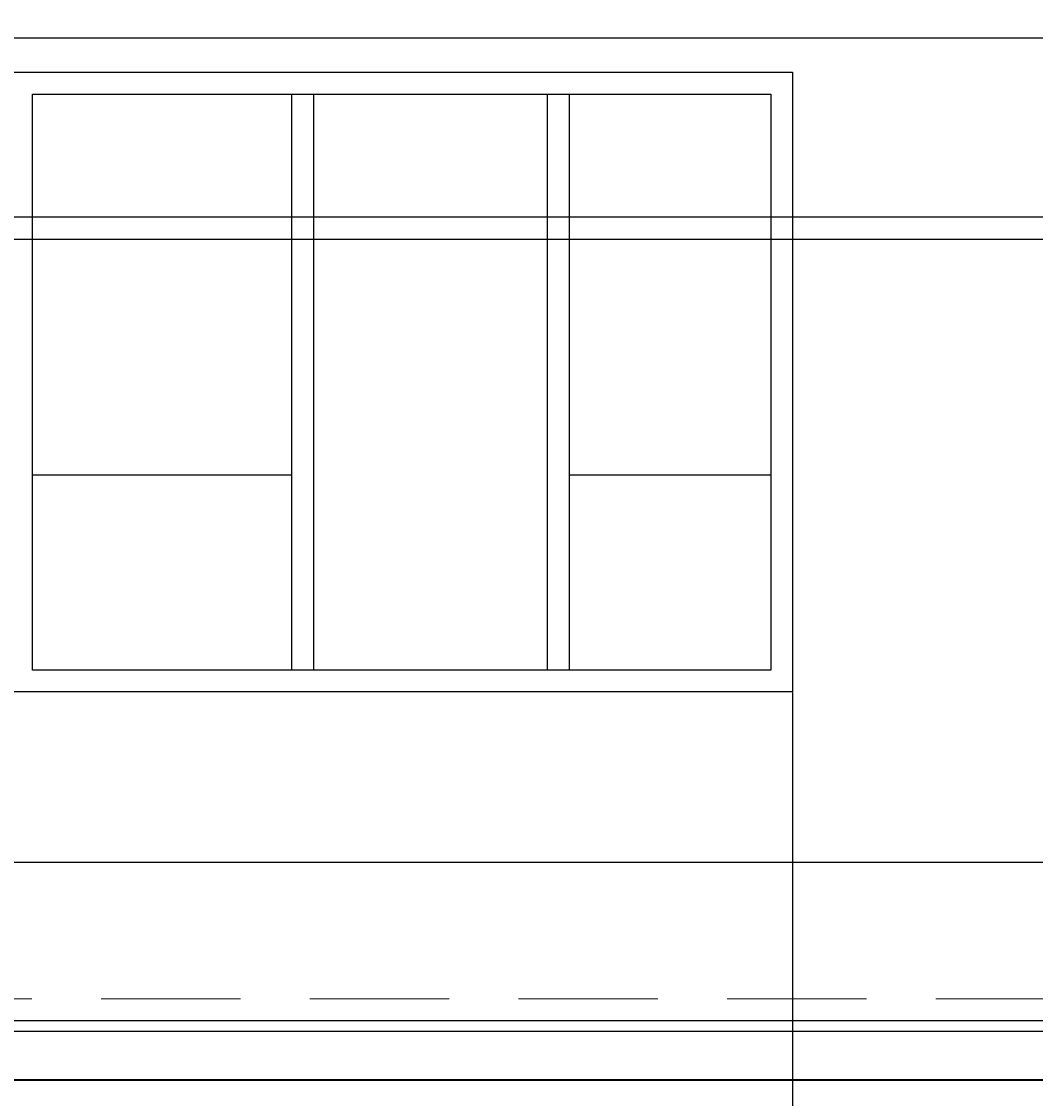
# Model space of a CAD drawing. Units: inches. Extents: x -145 to 510, y 5 to 386.
# Tile 6 of 25: x 89 to 182, y 78 to 177. Entities that reach past the tile are written whole.
import ezdxf

# ---------------------------------------------------------------- set-up
doc = ezdxf.new("R2010")
doc.units = ezdxf.units.IN
doc.header["$MEASUREMENT"] = 0
doc.linetypes.add('DASHED', pattern=[19.05, 12.7, -6.35])
for name, color, linetype, lineweight in [('A-ANNO-DIMS', 2, 'Continuous', 18), ('A-ELEV', 7, 'Continuous', 35), ('A-ELEV-HIDN', 8, 'DASHED', 18), ('A-GLAZ', 4, 'Continuous', 25)]:
    doc.layers.add(name, color=color, linetype=linetype, lineweight=lineweight)
doc.styles.get("Standard").update_dxf_attribs({"font": 'arial.ttf'})
doc.dimstyles.get("Standard").update_dxf_attribs({"dimtxt": 0.6875, "dimasz": 0.18, "dimexe": 0.18, "dimexo": 0.0625, "dimgap": 0.09, "dimtad": 0, "dimtih": 1, "dimtoh": 1, "dimdec": 4, "dimzin": 0, "dimdsep": 46, "dimlunit": 4, "dimtxsty": 'Standard', "dimcen": 0.09, "dimadec": 0, "dimazin": 0, "dimtfac": 1, "dimtdec": 4, "dimtofl": 0, "dimtmove": 0, "dimatfit": 3, "dimfxl": 1, "dimtolj": 1, "dimtzin": 0, "dimarcsym": 0})

# ---------------------------------------------------------------- blocks, each defined once
blk = doc.blocks.new('*D8')
at = {"layer": 'A-ANNO-DIMS', "color": 0, "lineweight": -2, "transparency": 16777216}
for p, q in [((88.246, 115.23), (88.246, 5.194)), ((159.649, 115.23), (159.649, 5.194)), ((88.426, 5.374), (122.969, 5.374)), ((159.469, 5.374), (124.926, 5.374))]:
    blk.add_line(p, q, dxfattribs=at)
at = {"layer": 'A-ANNO-DIMS', "color": 0, "transparency": 16777216}
for points in [[(88.426, 5.404), (88.426, 5.344), (88.246, 5.374)], [(159.469, 5.404), (159.469, 5.344), (159.649, 5.374)]]:
    blk.add_solid(points, dxfattribs=at)
at = {"layer": 'Defpoints', "color": 0, "transparency": 16777216}
for p in [(88.246, 115.292), (159.649, 115.292), (159.649, 5.374)]:
    blk.add_point(p, dxfattribs=at)
at = {"layer": 'A-ANNO-DIMS', "color": 0, "transparency": 16777216, "insert": (123.948, 5.374), "char_height": 0.6875, "attachment_point": 5}
blk.add_mtext('\\A1;71.4', dxfattribs=at)
blk = doc.blocks.new('*D9')
at = {"layer": 'A-ANNO-DIMS', "color": 0, "lineweight": -2, "transparency": 16777216}
for p, q in [((159.649, 115.23), (159.649, 5.194)), ((221.529, 85.201), (221.529, 5.194)), ((159.829, 5.374), (189.337, 5.374)), ((221.349, 5.374), (191.842, 5.374))]:
    blk.add_line(p, q, dxfattribs=at)
at = {"layer": 'A-ANNO-DIMS', "color": 0, "transparency": 16777216}
for points in [[(159.829, 5.404), (159.829, 5.344), (159.649, 5.374)], [(221.349, 5.404), (221.349, 5.344), (221.529, 5.374)]]:
    blk.add_solid(points, dxfattribs=at)
at = {"layer": 'Defpoints', "color": 0, "transparency": 16777216}
for p in [(159.649, 115.292), (221.529, 85.264), (221.529, 5.374)]:
    blk.add_point(p, dxfattribs=at)
at = {"layer": 'A-ANNO-DIMS', "color": 0, "transparency": 16777216, "insert": (190.589, 5.374), "char_height": 0.6875, "attachment_point": 5}
blk.add_mtext('\\A1;61.88', dxfattribs=at)
blk = doc.blocks.new('*D19')
at = {"layer": 'A-ANNO-DIMS', "color": 0, "lineweight": -2, "transparency": 16777216}
for p, q in [((478.764, 355.891), (-144.054, 355.891)), ((-143.874, 355.711), (-143.874, 218.332)), ((-143.874, 80.071), (-143.874, 217.45)), ((-114.036, 79.891), (-144.054, 79.891))]:
    blk.add_line(p, q, dxfattribs=at)
at = {"layer": 'A-ANNO-DIMS', "color": 0, "transparency": 16777216}
for points in [[(-143.904, 355.711), (-143.844, 355.711), (-143.874, 355.891)], [(-143.904, 80.071), (-143.844, 80.071), (-143.874, 79.891)]]:
    blk.add_solid(points, dxfattribs=at)
at = {"layer": 'Defpoints', "color": 0, "transparency": 16777216}
for p in [(-143.874, 355.891), (478.826, 355.891), (-113.974, 79.891)]:
    blk.add_point(p, dxfattribs=at)
at = {"layer": 'A-ANNO-DIMS', "color": 0, "transparency": 16777216, "insert": (-143.874, 217.891), "char_height": 0.6875, "attachment_point": 5}
blk.add_mtext('\\A1;276', dxfattribs=at)
blk = doc.blocks.new('*D29')
at = {"layer": 'A-ANNO-DIMS', "color": 0, "lineweight": -2, "transparency": 16777216}
for p, q in [((221.467, 174.992), (-144.054, 174.992)), ((-143.874, 174.812), (-143.874, 130.569)), ((-143.874, 85.444), (-143.874, 129.687)), ((221.467, 85.264), (-144.054, 85.264))]:
    blk.add_line(p, q, dxfattribs=at)
at = {"layer": 'A-ANNO-DIMS', "color": 0, "transparency": 16777216}
for points in [[(-143.904, 174.812), (-143.844, 174.812), (-143.874, 174.992)], [(-143.904, 85.444), (-143.844, 85.444), (-143.874, 85.264)]]:
    blk.add_solid(points, dxfattribs=at)
at = {"layer": 'Defpoints', "color": 0, "transparency": 16777216}
for p in [(-143.874, 174.992), (221.529, 174.992), (221.529, 85.264)]:
    blk.add_point(p, dxfattribs=at)
at = {"layer": 'A-ANNO-DIMS', "color": 0, "transparency": 16777216, "insert": (-143.874, 130.128), "char_height": 0.6875, "attachment_point": 5}
blk.add_mtext('\\A1;89.73', dxfattribs=at)
blk = doc.blocks.new('*D54')
at = {"layer": 'A-ANNO-DIMS', "color": 0, "lineweight": -2, "transparency": 16777216}
for p, q in [((315.492, 156.609), (-144.054, 156.609)), ((-143.874, 156.429), (-143.874, 121.378)), ((-143.874, 85.444), (-143.874, 120.495)), ((315.492, 85.264), (-144.054, 85.264))]:
    blk.add_line(p, q, dxfattribs=at)
at = {"layer": 'A-ANNO-DIMS', "color": 0, "transparency": 16777216}
for points in [[(-143.904, 156.429), (-143.844, 156.429), (-143.874, 156.609)], [(-143.904, 85.444), (-143.844, 85.444), (-143.874, 85.264)]]:
    blk.add_solid(points, dxfattribs=at)
at = {"layer": 'Defpoints', "color": 0, "transparency": 16777216}
for p in [(-143.874, 156.609), (315.554, 156.609), (315.554, 85.264)]:
    blk.add_point(p, dxfattribs=at)
at = {"layer": 'A-ANNO-DIMS', "color": 0, "transparency": 16777216, "insert": (-143.874, 120.937), "char_height": 0.6875, "attachment_point": 5}
blk.add_mtext('\\A1;71.35', dxfattribs=at)
blk = doc.blocks.new('*D55')
at = {"layer": 'A-ANNO-DIMS', "color": 0, "lineweight": -2, "transparency": 16777216}
for p, q in [((314.432, 174.992), (-144.054, 174.992)), ((-143.874, 174.812), (-143.874, 167.266)), ((-143.874, 158.837), (-143.874, 166.383)), ((314.432, 158.657), (-144.054, 158.657))]:
    blk.add_line(p, q, dxfattribs=at)
at = {"layer": 'A-ANNO-DIMS', "color": 0, "transparency": 16777216}
for points in [[(-143.904, 174.812), (-143.844, 174.812), (-143.874, 174.992)], [(-143.904, 158.837), (-143.844, 158.837), (-143.874, 158.657)]]:
    blk.add_solid(points, dxfattribs=at)
at = {"layer": 'Defpoints', "color": 0, "transparency": 16777216}
for p in [(-143.874, 174.992), (314.494, 174.992), (314.494, 158.657)]:
    blk.add_point(p, dxfattribs=at)
at = {"layer": 'A-ANNO-DIMS', "color": 0, "transparency": 16777216, "insert": (-143.874, 166.825), "char_height": 0.6875, "attachment_point": 5}
blk.add_mtext('\\A1;16.335', dxfattribs=at)
blk = doc.blocks.new('*D57')
at = {"layer": 'A-ANNO-DIMS', "color": 0, "lineweight": -2, "transparency": 16777216}
for p, q in [((263.856, 99.712), (-144.054, 99.712)), ((-143.874, 99.532), (-143.874, 92.436)), ((-143.874, 84.459), (-143.874, 91.554)), ((271.428, 84.279), (-144.054, 84.279))]:
    blk.add_line(p, q, dxfattribs=at)
at = {"layer": 'A-ANNO-DIMS', "color": 0, "transparency": 16777216}
for points in [[(-143.904, 99.532), (-143.844, 99.532), (-143.874, 99.712)], [(-143.904, 84.459), (-143.844, 84.459), (-143.874, 84.279)]]:
    blk.add_solid(points, dxfattribs=at)
at = {"layer": 'Defpoints', "color": 0, "transparency": 16777216}
for p in [(-143.874, 99.712), (263.918, 99.712), (271.491, 84.279)]:
    blk.add_point(p, dxfattribs=at)
at = {"layer": 'A-ANNO-DIMS', "color": 0, "transparency": 16777216, "insert": (-143.874, 91.995), "char_height": 0.6875, "attachment_point": 5}
blk.add_mtext('\\A1;15.433', dxfattribs=at)

msp = doc.modelspace()

# ---------------------------------------------------------------- linework, layer by layer
at = {"layer": 'A-ELEV'}
msp.add_line((54.0014, 79.8905), (392.4492, 79.8905), dxfattribs=at)
at = {"layer": 'A-ELEV-HIDN'}
msp.add_line((223.5292, 87.2638), (54.0014, 87.2638), dxfattribs=at)
at = {"layer": 'A-GLAZ'}
for p, q in [((113.8964, 169.8717), (113.8964, 117.2922)), ((115.8964, 169.8717), (115.8964, 117.2922)), ((137.2509, 169.8717), (137.2509, 117.2922)), ((139.2509, 169.8717), (139.2509, 117.2922)), ((90.2462, 135.1151), (113.8964, 135.1151)), ((139.2509, 135.1151), (157.6492, 135.1151))]:
    msp.add_line(p, q, dxfattribs=at)
for points in [[(88.2462, 171.8717), (159.6492, 171.8717), (159.6492, 115.2922), (88.2462, 115.2922)], [(90.2462, 169.8717), (157.6492, 169.8717), (157.6492, 117.2922), (90.2462, 117.2922)]]:
    msp.add_lwpolyline(points, close=True, dxfattribs=at)

# ---------------------------------------------------------------- dimensions: what is measured, and where the dimension line sits
at = {"layer": 'A-ANNO-DIMS'}
for base, p1, p2, override, picture, middle in [((-143.8737, 355.8905), (-113.9737, 79.8905), (478.8263, 355.8905), {"dimdec": 0, "dimlfac": 1, "dimrnd": 0, "dimzin": 0, "dimdsep": 46, "dimlunit": 2}, '*D19', (-143.8737, 217.8905)), ((-143.8737, 174.9923), (314.494, 158.657), (314.494, 174.9923), {"dimdec": 3, "dimlfac": 1, "dimrnd": 0, "dimzin": 0, "dimdsep": 46, "dimlunit": 2}, '*D55', (-143.8737, 166.8247)), ((-143.8737, 174.9923), (221.5292, 85.2638), (221.5292, 174.9923), {"dimdec": 2, "dimlfac": 1, "dimrnd": 0, "dimzin": 0, "dimdsep": 46, "dimlunit": 2}, '*D29', (-143.8737, 130.1281)), ((-143.8737, 156.6093), (315.5545, 85.2638), (315.5545, 156.6093), {"dimdec": 2, "dimlfac": 1, "dimrnd": 0, "dimzin": 0, "dimdsep": 46, "dimlunit": 2}, '*D54', (-143.8737, 120.9365)), ((-143.8737, 99.7118), (271.4905, 84.2785), (263.9183, 99.7118), {"dimdec": 3, "dimlfac": 1, "dimrnd": 0, "dimzin": 0, "dimdsep": 46, "dimlunit": 2}, '*D57', (-143.8737, 91.9952))]:
    dim = msp.add_linear_dim(base=base, p1=p1, p2=p2, angle=90, dimstyle='Standard', override=override, dxfattribs=at)
    dim.commit()
    dim.dimension.update_dxf_attribs({"geometry": picture, "text_midpoint": middle})
for base, p1, p2, override, picture, middle in [((159.6492, 5.3738), (88.2462, 115.2922), (159.6492, 115.2922), {"dimdec": 1, "dimlfac": 1, "dimrnd": 0, "dimzin": 0, "dimdsep": 46, "dimlunit": 2}, '*D8', (123.9477, 5.3738)), ((221.5292, 5.3738), (159.6492, 115.2922), (221.5292, 85.2638), {"dimdec": 2, "dimlfac": 1, "dimrnd": 0, "dimzin": 0, "dimdsep": 46, "dimlunit": 2}, '*D9', (190.5892, 5.3738))]:
    dim = msp.add_linear_dim(base=base, p1=p1, p2=p2, dimstyle='Standard', override=override, dxfattribs=at)
    dim.commit()
    dim.dimension.update_dxf_attribs({"geometry": picture, "text_midpoint": middle})

doc.saveas('drawing.dxf')
